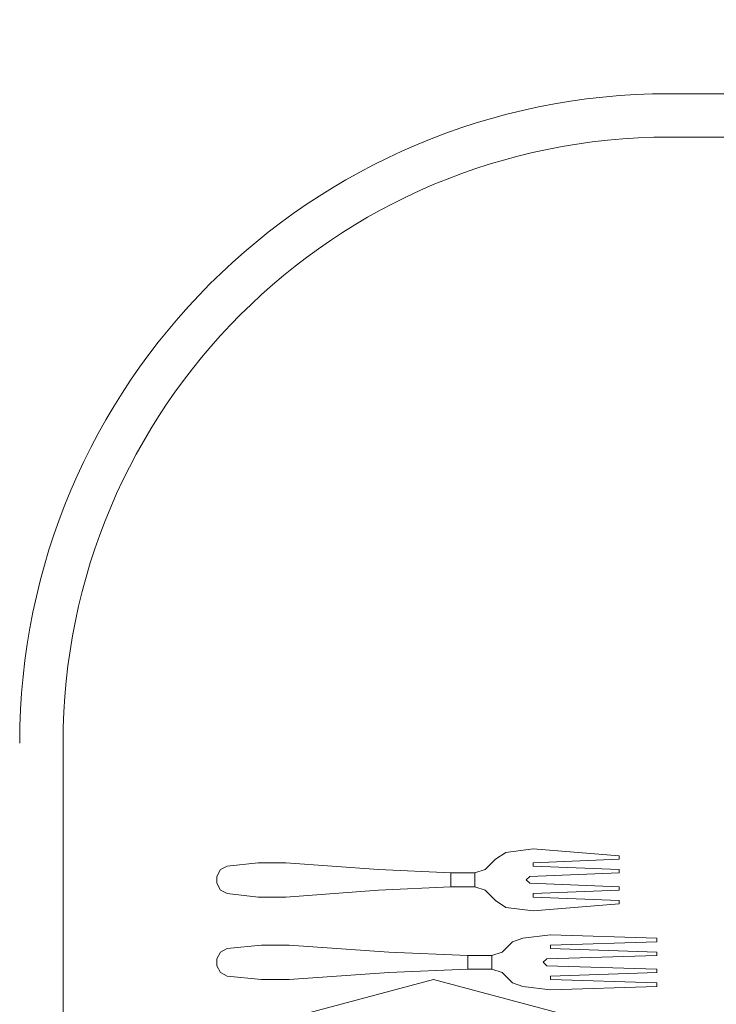
# Model space of a CAD drawing. Units: inches. Extents: x 375 to 1122, y 27 to 1069.
# Tile 46 of 155: x 705.14 to 717.62, y 308.18 to 325.82. Entities that reach past the tile are written whole.
import ezdxf

# ---------------------------------------------------------------- set-up
doc = ezdxf.new("R2010")
doc.units = ezdxf.units.IN
doc.layers.add('A-ANNO-DIMS', color=2, linetype='Continuous', lineweight=18)
doc.layers.add('Furniture', color=30, linetype='Continuous', lineweight=18)
doc.styles.get("Standard").update_dxf_attribs({"font": 'arial.ttf'})
doc.dimstyles.new('ISO-25', dxfattribs={"dimtxt": 12, "dimasz": 2.5, "dimexe": 1.5, "dimexo": 1.5, "dimtad": 1, "dimdec": 1, "dimlunit": 3, "dimtxsty": 'Standard', "dimblk": 'ARCHTICK', "dimcen": 2.5, "dimadec": 0, "dimazin": 0, "dimtfac": 1, "dimtdec": 1, "dimtmove": 0, "dimatfit": 3, "dimfxl": 1.5, "dimfxlon": 1, "dimarcsym": 0})

# ---------------------------------------------------------------- blocks, each defined once
blk = doc.blocks.new('A$C403C54AD')
for p, q in [((0.54488, 0.79569, -0.0006), (0.54488, 1.26108, -0.0006)), ((0.56427, 0.79569, -0.0006), (0.56427, 1.26108, -0.0006)), ((0.92321, 0.73013, -0.02105), (0.92475, 0.72551, -0.02059)), ((0.92321, 0.73013, -0.02413), (0.92475, 0.72551, -0.02367)), ((0.88473, 0.72244, -0.02105), (0.88781, 0.71782, -0.02059)), ((0.88473, 0.72244, -0.02413), (0.88781, 0.71782, -0.02367)), ((0.83575, 0.52421, -0.0006), (1.99923, 0.52421, -0.0006))]:
    blk.add_line(p, q)
for radius in [0.29087, 0.27148]:
    blk.add_arc((0.83575, 0.79569, -0.0006), radius, 180, 270)
for points, invisible_edges in [([(0.92629, 0.74244, -0.02045), (0.92167, 0.74244, -0.02045), (0.92321, 0.79016, -0.01335), (0.92475, 0.79016, -0.01335)], 1), ([(0.92629, 0.74244, -0.02353), (0.92167, 0.74244, -0.02353), (0.92321, 0.79016, -0.01643), (0.92475, 0.79016, -0.01643)], 1), ([(0.93244, 0.74091, -0.0207), (0.92782, 0.74244, -0.02045), (0.92936, 0.79016, -0.01335), (0.9309, 0.79016, -0.01335)], 1), ([(0.93244, 0.74091, -0.02378), (0.92782, 0.74244, -0.02353), (0.92936, 0.79016, -0.01643), (0.9309, 0.79016, -0.01643)], 1), ([(0.94014, 0.74244, -0.02045), (0.93552, 0.74091, -0.0207), (0.93706, 0.79016, -0.01335), (0.9386, 0.79016, -0.01335)], 1), ([(0.94014, 0.74244, -0.02353), (0.93552, 0.74091, -0.02378), (0.93706, 0.79016, -0.01643), (0.9386, 0.79016, -0.01643)], 1), ([(0.94168, 0.74244, -0.02045), (0.9463, 0.74244, -0.02045), (0.94476, 0.79016, -0.01335), (0.94322, 0.79016, -0.01335)], 1), ([(0.94168, 0.74244, -0.02353), (0.9463, 0.74244, -0.02353), (0.94476, 0.79016, -0.01643), (0.94322, 0.79016, -0.01643)], 1), ([(0.88935, 0.73475, -0.02045), (0.88319, 0.73475, -0.02045), (0.88627, 0.77323, -0.01335), (0.88781, 0.77323, -0.01335)], 1), ([(0.88935, 0.73475, -0.02353), (0.88319, 0.73475, -0.02353), (0.88627, 0.77323, -0.01643), (0.88781, 0.77323, -0.01643)], 1), ([(0.8955, 0.73321, -0.0207), (0.89088, 0.73475, -0.02045), (0.89242, 0.77323, -0.01335), (0.89396, 0.77323, -0.01335)], 1), ([(0.8955, 0.73321, -0.02378), (0.89088, 0.73475, -0.02353), (0.89242, 0.77323, -0.01643), (0.89396, 0.77323, -0.01643)], 1), ([(0.9032, 0.73475, -0.02045), (0.89858, 0.73321, -0.0207), (0.90012, 0.77323, -0.01335), (0.90166, 0.77323, -0.01335)], 1), ([(0.9032, 0.73475, -0.02353), (0.89858, 0.73321, -0.02378), (0.90012, 0.77323, -0.01643), (0.90166, 0.77323, -0.01643)], 1), ([(0.90474, 0.73475, -0.02045), (0.91089, 0.73475, -0.02045), (0.90782, 0.77323, -0.01335), (0.90628, 0.77323, -0.01335)], 1), ([(0.90474, 0.73475, -0.02353), (0.91089, 0.73475, -0.02353), (0.90782, 0.77323, -0.01643), (0.90628, 0.77323, -0.01643)], 1), ([(0.92321, 0.73013, -0.02105), (0.92782, 0.74244, -0.02045), (0.92629, 0.74244, -0.02045), (0.92167, 0.74244, -0.02045)], 5), ([(0.92321, 0.73013, -0.02413), (0.92782, 0.74244, -0.02353), (0.92629, 0.74244, -0.02353), (0.92167, 0.74244, -0.02353)], 5), ([(0.92321, 0.73013, -0.02413), (0.92321, 0.73013, -0.02105), (0.92167, 0.74244, -0.02045), (0.92167, 0.74244, -0.02353)], 1), ([(0.92321, 0.73013, -0.02105), (0.93398, 0.73924, -0.02085), (0.93244, 0.74091, -0.0207), (0.92782, 0.74244, -0.02045)], 13), ([(0.92321, 0.73013, -0.02413), (0.93398, 0.73924, -0.02392), (0.93244, 0.74091, -0.02378), (0.92782, 0.74244, -0.02353)], 13), ([(0.94476, 0.73013, -0.02105), (0.93398, 0.73924, -0.02085), (0.93552, 0.74091, -0.0207), (0.94014, 0.74244, -0.02045)], 13), ([(0.94476, 0.73013, -0.02413), (0.93398, 0.73924, -0.02392), (0.93552, 0.74091, -0.02378), (0.94014, 0.74244, -0.02353)], 13), ([(0.94476, 0.73013, -0.02105), (0.94014, 0.74244, -0.02045), (0.94168, 0.74244, -0.02045), (0.9463, 0.74244, -0.02045)], 5), ([(0.94476, 0.73013, -0.02413), (0.94014, 0.74244, -0.02353), (0.94168, 0.74244, -0.02353), (0.9463, 0.74244, -0.02353)], 5), ([(0.94476, 0.73013, -0.02105), (0.94476, 0.73013, -0.02413), (0.9463, 0.74244, -0.02353), (0.9463, 0.74244, -0.02045)], 1), ([(0.94476, 0.73013, -0.02105), (0.93398, 0.73924, -0.02085), (0.92321, 0.73013, -0.02105), (0.94476, 0.73013, -0.02105)], 7), ([(0.94476, 0.73013, -0.02413), (0.93398, 0.73924, -0.02392), (0.92321, 0.73013, -0.02413), (0.94476, 0.73013, -0.02413)], 7), ([(0.88473, 0.72244, -0.02105), (0.89088, 0.73475, -0.02045), (0.88935, 0.73475, -0.02045), (0.88319, 0.73475, -0.02045)], 5), ([(0.88473, 0.72244, -0.02413), (0.89088, 0.73475, -0.02353), (0.88935, 0.73475, -0.02353), (0.88319, 0.73475, -0.02353)], 5), ([(0.88473, 0.72244, -0.02413), (0.88473, 0.72244, -0.02105), (0.88319, 0.73475, -0.02045), (0.88319, 0.73475, -0.02353)], 1), ([(0.88473, 0.72244, -0.02105), (0.89704, 0.73155, -0.02085), (0.8955, 0.73321, -0.0207), (0.89088, 0.73475, -0.02045)], 13), ([(0.88473, 0.72244, -0.02413), (0.89704, 0.73155, -0.02392), (0.8955, 0.73321, -0.02378), (0.89088, 0.73475, -0.02353)], 13), ([(0.90935, 0.72244, -0.02105), (0.89704, 0.73155, -0.02085), (0.89858, 0.73321, -0.0207), (0.9032, 0.73475, -0.02045)], 13), ([(0.90935, 0.72244, -0.02413), (0.89704, 0.73155, -0.02392), (0.89858, 0.73321, -0.02378), (0.9032, 0.73475, -0.02353)], 13), ([(0.90935, 0.72244, -0.02105), (0.9032, 0.73475, -0.02045), (0.90474, 0.73475, -0.02045), (0.91089, 0.73475, -0.02045)], 5), ([(0.90935, 0.72244, -0.02413), (0.9032, 0.73475, -0.02353), (0.90474, 0.73475, -0.02353), (0.91089, 0.73475, -0.02353)], 5), ([(0.90935, 0.72244, -0.02105), (0.90935, 0.72244, -0.02413), (0.91089, 0.73475, -0.02353), (0.91089, 0.73475, -0.02045)], 1), ([(0.90935, 0.72244, -0.02105), (0.89704, 0.73155, -0.02085), (0.88473, 0.72244, -0.02105), (0.90935, 0.72244, -0.02105)], 7), ([(0.90935, 0.72244, -0.02413), (0.89704, 0.73155, -0.02392), (0.88473, 0.72244, -0.02413), (0.90935, 0.72244, -0.02413)], 7), ([(0.94322, 0.72551, -0.02059), (0.92475, 0.72551, -0.02059), (0.92321, 0.73013, -0.02105), (0.94476, 0.73013, -0.02105)], 5), ([(0.94322, 0.72551, -0.02367), (0.92475, 0.72551, -0.02367), (0.92321, 0.73013, -0.02413), (0.94476, 0.73013, -0.02413)], 5), ([(0.92475, 0.72551, -0.02059), (0.92475, 0.72551, -0.02367), (0.92321, 0.73013, -0.02413), (0.92321, 0.73013, -0.02105)], 4), ([(0.94322, 0.72551, -0.02367), (0.94322, 0.72551, -0.02059), (0.94476, 0.73013, -0.02105), (0.94476, 0.73013, -0.02413)], 4), ([(0.92782, 0.72244, -0.02243), (0.94014, 0.72244, -0.02243), (0.94322, 0.72551, -0.02367), (0.92475, 0.72551, -0.02367)], 5), ([(0.92782, 0.72244, -0.01935), (0.94014, 0.72244, -0.01935), (0.94322, 0.72551, -0.02059), (0.92475, 0.72551, -0.02059)], 5), ([(0.90628, 0.71782, -0.02059), (0.88781, 0.71782, -0.02059), (0.88473, 0.72244, -0.02105), (0.90935, 0.72244, -0.02105)], 5), ([(0.90628, 0.71782, -0.02367), (0.88781, 0.71782, -0.02367), (0.88473, 0.72244, -0.02413), (0.90935, 0.72244, -0.02413)], 5), ([(0.88781, 0.71782, -0.02059), (0.88781, 0.71782, -0.02367), (0.88473, 0.72244, -0.02413), (0.88473, 0.72244, -0.02105)], 4), ([(0.90628, 0.71782, -0.02367), (0.90628, 0.71782, -0.02059), (0.90935, 0.72244, -0.02105), (0.90935, 0.72244, -0.02413)], 4), ([(0.92936, 0.7209, -0.0183), (0.9386, 0.7209, -0.0183), (0.94014, 0.72244, -0.01935), (0.92782, 0.72244, -0.01935)], 5), ([(0.92936, 0.7209, -0.02109), (0.9386, 0.7209, -0.02109), (0.94014, 0.72244, -0.02243), (0.92782, 0.72244, -0.02243)], 5), ([(0.92936, 0.7209, -0.0183), (0.92936, 0.7209, -0.02109), (0.92782, 0.72244, -0.02243), (0.92782, 0.72244, -0.01935)], 1), ([(0.93706, 0.71628, -0.01595), (0.9309, 0.71628, -0.01595), (0.92936, 0.7209, -0.0183), (0.9386, 0.7209, -0.0183)], 4), ([(0.9309, 0.71628, -0.01854), (0.9309, 0.71628, -0.01595), (0.92936, 0.7209, -0.0183), (0.92936, 0.7209, -0.02109)], 5), ([(0.93706, 0.71628, -0.01854), (0.9309, 0.71628, -0.01854), (0.92936, 0.7209, -0.02109), (0.9386, 0.7209, -0.02109)], 4), ([(0.93706, 0.71628, -0.01595), (0.93706, 0.71628, -0.01854), (0.9386, 0.7209, -0.02109), (0.9386, 0.7209, -0.0183)], 5), ([(0.9386, 0.7209, -0.02109), (0.9386, 0.7209, -0.0183), (0.94014, 0.72244, -0.01935), (0.94014, 0.72244, -0.02243)], 1), ([(0.89088, 0.71474, -0.02243), (0.9032, 0.71474, -0.02243), (0.90628, 0.71782, -0.02367), (0.88781, 0.71782, -0.02367)], 5), ([(0.89088, 0.71474, -0.01935), (0.9032, 0.71474, -0.01935), (0.90628, 0.71782, -0.02059), (0.88781, 0.71782, -0.02059)], 5), ([(0.89242, 0.7132, -0.0183), (0.90166, 0.7132, -0.0183), (0.9032, 0.71474, -0.01935), (0.89088, 0.71474, -0.01935)], 5), ([(0.89242, 0.7132, -0.02109), (0.90166, 0.7132, -0.02109), (0.9032, 0.71474, -0.02243), (0.89088, 0.71474, -0.02243)], 5), ([(0.89242, 0.7132, -0.0183), (0.89242, 0.7132, -0.02109), (0.89088, 0.71474, -0.02243), (0.89088, 0.71474, -0.01935)], 1), ([(0.90166, 0.7132, -0.02109), (0.90166, 0.7132, -0.0183), (0.9032, 0.71474, -0.01935), (0.9032, 0.71474, -0.02243)], 1), ([(0.9309, 0.71628, -0.01854), (0.9309, 0.71628, -0.01595), (0.9309, 0.7055, -0.01387), (0.9309, 0.7055, -0.01646)], 5), ([(0.93706, 0.7055, -0.01646), (0.93706, 0.7055, -0.01387), (0.93706, 0.71628, -0.01595), (0.93706, 0.71628, -0.01854)], 5), ([(0.90012, 0.70858, -0.01595), (0.89396, 0.70858, -0.01595), (0.89242, 0.7132, -0.0183), (0.90166, 0.7132, -0.0183)], 4), ([(0.90012, 0.70858, -0.01854), (0.89396, 0.70858, -0.01854), (0.89242, 0.7132, -0.02109), (0.90166, 0.7132, -0.02109)], 4), ([(0.89396, 0.70858, -0.01854), (0.89396, 0.70858, -0.01595), (0.89242, 0.7132, -0.0183), (0.89242, 0.7132, -0.02109)], 5), ([(0.90012, 0.70858, -0.01595), (0.90012, 0.70858, -0.01854), (0.90166, 0.7132, -0.02109), (0.90166, 0.7132, -0.0183)], 5), ([(0.89396, 0.70858, -0.01854), (0.89396, 0.70858, -0.01595), (0.89396, 0.69781, -0.01387), (0.89396, 0.69781, -0.01646)], 5), ([(0.90012, 0.69781, -0.01646), (0.90012, 0.69781, -0.01387), (0.90012, 0.70858, -0.01595), (0.90012, 0.70858, -0.01854)], 5), ([(0.9386, 0.6701, -0.01678), (0.92936, 0.6701, -0.01678), (0.9309, 0.7055, -0.01387), (0.93706, 0.7055, -0.01387)], 1), ([(0.9309, 0.7055, -0.01387), (0.9309, 0.7055, -0.01646), (0.92936, 0.6701, -0.01986), (0.92936, 0.6701, -0.01678)], 5), ([(0.9386, 0.6701, -0.01986), (0.92936, 0.6701, -0.01986), (0.9309, 0.7055, -0.01646), (0.93706, 0.7055, -0.01646)], 1), ([(0.9386, 0.6701, -0.01678), (0.9386, 0.6701, -0.01986), (0.93706, 0.7055, -0.01646), (0.93706, 0.7055, -0.01387)], 5), ([(0.90166, 0.66549, -0.01678), (0.89242, 0.66549, -0.01678), (0.89396, 0.69781, -0.01387), (0.90012, 0.69781, -0.01387)], 1), ([(0.89396, 0.69781, -0.01387), (0.89396, 0.69781, -0.01646), (0.89242, 0.66549, -0.01986), (0.89242, 0.66549, -0.01678)], 5), ([(0.90166, 0.66549, -0.01986), (0.89242, 0.66549, -0.01986), (0.89396, 0.69781, -0.01646), (0.90012, 0.69781, -0.01646)], 1), ([(0.90166, 0.66549, -0.01678), (0.90166, 0.66549, -0.01986), (0.90012, 0.69781, -0.01646), (0.90012, 0.69781, -0.01387)], 5), ([(0.92629, 0.62547, -0.01916), (0.94168, 0.62547, -0.01916), (0.9386, 0.6701, -0.01678), (0.92936, 0.6701, -0.01678)], 5), ([(0.92629, 0.62547, -0.0238), (0.94168, 0.62547, -0.0238), (0.9386, 0.6701, -0.01986), (0.92936, 0.6701, -0.01986)], 5), ([(0.92936, 0.6701, -0.01986), (0.92936, 0.6701, -0.01678), (0.92629, 0.62547, -0.01916), (0.92629, 0.62547, -0.0238)], 1), ([(0.94168, 0.62547, -0.0238), (0.94168, 0.62547, -0.01916), (0.9386, 0.6701, -0.01678), (0.9386, 0.6701, -0.01986)], 4), ([(0.88935, 0.62393, -0.01916), (0.90474, 0.62393, -0.01916), (0.90166, 0.66549, -0.01678), (0.89242, 0.66549, -0.01678)], 5), ([(0.88935, 0.62393, -0.0238), (0.90474, 0.62393, -0.0238), (0.90166, 0.66549, -0.01986), (0.89242, 0.66549, -0.01986)], 5), ([(0.89242, 0.66549, -0.01986), (0.89242, 0.66549, -0.01678), (0.88935, 0.62393, -0.01916), (0.88935, 0.62393, -0.0238)], 1), ([(0.90474, 0.62393, -0.0238), (0.90474, 0.62393, -0.01916), (0.90166, 0.66549, -0.01678), (0.90166, 0.66549, -0.01986)], 4), ([(0.90474, 0.61161, -0.01949), (0.88935, 0.61161, -0.01949), (0.88935, 0.62393, -0.01916), (0.90474, 0.62393, -0.01916)], 5), ([(0.90474, 0.61161, -0.02413), (0.88935, 0.61161, -0.02413), (0.88935, 0.62393, -0.0238), (0.90474, 0.62393, -0.0238)], 5), ([(0.94168, 0.61315, -0.01949), (0.92629, 0.61315, -0.01949), (0.92629, 0.62547, -0.01916), (0.94168, 0.62547, -0.01916)], 5), ([(0.94168, 0.61315, -0.02413), (0.92629, 0.61315, -0.02413), (0.92629, 0.62547, -0.0238), (0.94168, 0.62547, -0.0238)], 5), ([(0.92782, 0.59776, -0.01946), (0.94014, 0.59776, -0.01946), (0.94168, 0.61315, -0.01949), (0.92629, 0.61315, -0.01949)], 5), ([(0.92782, 0.59776, -0.02409), (0.94014, 0.59776, -0.02409), (0.94168, 0.61315, -0.02413), (0.92629, 0.61315, -0.02413)], 5), ([(0.89088, 0.59776, -0.01946), (0.9032, 0.59776, -0.01946), (0.90474, 0.61161, -0.01949), (0.88935, 0.61161, -0.01949)], 5), ([(0.89088, 0.59776, -0.02409), (0.9032, 0.59776, -0.02409), (0.90474, 0.61161, -0.02413), (0.88935, 0.61161, -0.02413)], 5), ([(0.90166, 0.59468, -0.01921), (0.89242, 0.59468, -0.01921), (0.89088, 0.59776, -0.01946), (0.9032, 0.59776, -0.01946)], 5), ([(0.90166, 0.59468, -0.02385), (0.89242, 0.59468, -0.02385), (0.89088, 0.59776, -0.02409), (0.9032, 0.59776, -0.02409)], 5), ([(0.9386, 0.59468, -0.01921), (0.92936, 0.59468, -0.01921), (0.92782, 0.59776, -0.01946), (0.94014, 0.59776, -0.01946)], 5), ([(0.9386, 0.59468, -0.02385), (0.92936, 0.59468, -0.02385), (0.92782, 0.59776, -0.02409), (0.94014, 0.59776, -0.02409)], 5), ([(0.8955, 0.59314, -0.01938), (0.89858, 0.59314, -0.01938), (0.90166, 0.59468, -0.01921), (0.89242, 0.59468, -0.01921)], 4), ([(0.8955, 0.59314, -0.02351), (0.89858, 0.59314, -0.02351), (0.90166, 0.59468, -0.02385), (0.89242, 0.59468, -0.02385)], 4), ([(0.93244, 0.59314, -0.01938), (0.93552, 0.59314, -0.01938), (0.9386, 0.59468, -0.01921), (0.92936, 0.59468, -0.01921)], 4), ([(0.93244, 0.59314, -0.02351), (0.93552, 0.59314, -0.02351), (0.9386, 0.59468, -0.02385), (0.92936, 0.59468, -0.02385)], 4)]:
    blk.add_3dface(points, dxfattribs=dict(invisible_edges=invisible_edges))
for points in [[(0.92321, 0.79016, -0.01335), (0.92321, 0.79016, -0.01643), (0.92167, 0.74244, -0.02353), (0.92167, 0.74244, -0.02045)], [(0.92475, 0.79016, -0.01643), (0.92475, 0.79016, -0.01335), (0.92321, 0.79016, -0.01335), (0.92321, 0.79016, -0.01643)], [(0.92629, 0.74244, -0.02045), (0.92629, 0.74244, -0.02353), (0.92475, 0.79016, -0.01643), (0.92475, 0.79016, -0.01335)], [(0.92936, 0.79016, -0.01335), (0.92936, 0.79016, -0.01643), (0.92782, 0.74244, -0.02353), (0.92782, 0.74244, -0.02045)], [(0.9309, 0.79016, -0.01643), (0.9309, 0.79016, -0.01335), (0.92936, 0.79016, -0.01335), (0.92936, 0.79016, -0.01643)], [(0.93244, 0.74091, -0.02378), (0.93244, 0.74091, -0.0207), (0.9309, 0.79016, -0.01335), (0.9309, 0.79016, -0.01643)], [(0.93706, 0.79016, -0.01643), (0.93706, 0.79016, -0.01335), (0.93552, 0.74091, -0.0207), (0.93552, 0.74091, -0.02378)], [(0.9386, 0.79016, -0.01643), (0.9386, 0.79016, -0.01335), (0.93706, 0.79016, -0.01335), (0.93706, 0.79016, -0.01643)], [(0.94014, 0.74244, -0.02353), (0.94014, 0.74244, -0.02045), (0.9386, 0.79016, -0.01335), (0.9386, 0.79016, -0.01643)], [(0.94322, 0.79016, -0.01335), (0.94322, 0.79016, -0.01643), (0.94168, 0.74244, -0.02353), (0.94168, 0.74244, -0.02045)], [(0.94476, 0.79016, -0.01643), (0.94476, 0.79016, -0.01335), (0.94322, 0.79016, -0.01335), (0.94322, 0.79016, -0.01643)], [(0.9463, 0.74244, -0.02353), (0.9463, 0.74244, -0.02045), (0.94476, 0.79016, -0.01335), (0.94476, 0.79016, -0.01643)], [(0.88627, 0.77323, -0.01335), (0.88627, 0.77323, -0.01643), (0.88319, 0.73475, -0.02353), (0.88319, 0.73475, -0.02045)], [(0.88781, 0.77323, -0.01643), (0.88781, 0.77323, -0.01335), (0.88627, 0.77323, -0.01335), (0.88627, 0.77323, -0.01643)], [(0.88935, 0.73475, -0.02045), (0.88935, 0.73475, -0.02353), (0.88781, 0.77323, -0.01643), (0.88781, 0.77323, -0.01335)], [(0.89242, 0.77323, -0.01335), (0.89242, 0.77323, -0.01643), (0.89088, 0.73475, -0.02353), (0.89088, 0.73475, -0.02045)], [(0.89396, 0.77323, -0.01643), (0.89396, 0.77323, -0.01335), (0.89242, 0.77323, -0.01335), (0.89242, 0.77323, -0.01643)], [(0.8955, 0.73321, -0.02378), (0.8955, 0.73321, -0.0207), (0.89396, 0.77323, -0.01335), (0.89396, 0.77323, -0.01643)], [(0.90012, 0.77323, -0.01643), (0.90012, 0.77323, -0.01335), (0.89858, 0.73321, -0.0207), (0.89858, 0.73321, -0.02378)], [(0.90166, 0.77323, -0.01643), (0.90166, 0.77323, -0.01335), (0.90012, 0.77323, -0.01335), (0.90012, 0.77323, -0.01643)], [(0.9032, 0.73475, -0.02353), (0.9032, 0.73475, -0.02045), (0.90166, 0.77323, -0.01335), (0.90166, 0.77323, -0.01643)], [(0.90628, 0.77323, -0.01335), (0.90628, 0.77323, -0.01643), (0.90474, 0.73475, -0.02353), (0.90474, 0.73475, -0.02045)], [(0.90782, 0.77323, -0.01643), (0.90782, 0.77323, -0.01335), (0.90628, 0.77323, -0.01335), (0.90628, 0.77323, -0.01643)], [(0.91089, 0.73475, -0.02353), (0.91089, 0.73475, -0.02045), (0.90782, 0.77323, -0.01335), (0.90782, 0.77323, -0.01643)], [(0.92629, 0.74244, -0.02045), (0.92629, 0.74244, -0.02353), (0.92782, 0.74244, -0.02353), (0.92782, 0.74244, -0.02045)], [(0.94014, 0.74244, -0.02353), (0.94014, 0.74244, -0.02045), (0.94168, 0.74244, -0.02045), (0.94168, 0.74244, -0.02353)], [(0.93244, 0.74091, -0.0207), (0.93244, 0.74091, -0.02378), (0.93398, 0.73924, -0.02392), (0.93398, 0.73924, -0.02085)], [(0.93398, 0.73924, -0.02392), (0.93398, 0.73924, -0.02085), (0.93552, 0.74091, -0.0207), (0.93552, 0.74091, -0.02378)], [(0.88935, 0.73475, -0.02045), (0.88935, 0.73475, -0.02353), (0.89088, 0.73475, -0.02353), (0.89088, 0.73475, -0.02045)], [(0.8955, 0.73321, -0.0207), (0.8955, 0.73321, -0.02378), (0.89704, 0.73155, -0.02392), (0.89704, 0.73155, -0.02085)], [(0.89704, 0.73155, -0.02392), (0.89704, 0.73155, -0.02085), (0.89858, 0.73321, -0.0207), (0.89858, 0.73321, -0.02378)], [(0.9032, 0.73475, -0.02353), (0.9032, 0.73475, -0.02045), (0.90474, 0.73475, -0.02045), (0.90474, 0.73475, -0.02353)], [(0.92782, 0.72244, -0.02243), (0.92782, 0.72244, -0.01935), (0.92475, 0.72551, -0.02059), (0.92475, 0.72551, -0.02367)], [(0.94014, 0.72244, -0.01935), (0.94014, 0.72244, -0.02243), (0.94322, 0.72551, -0.02367), (0.94322, 0.72551, -0.02059)], [(0.89088, 0.71474, -0.02243), (0.89088, 0.71474, -0.01935), (0.88781, 0.71782, -0.02059), (0.88781, 0.71782, -0.02367)], [(0.9032, 0.71474, -0.01935), (0.9032, 0.71474, -0.02243), (0.90628, 0.71782, -0.02367), (0.90628, 0.71782, -0.02059)], [(0.9309, 0.7055, -0.01387), (0.93706, 0.7055, -0.01387), (0.93706, 0.71628, -0.01595), (0.9309, 0.71628, -0.01595)], [(0.9309, 0.7055, -0.01646), (0.93706, 0.7055, -0.01646), (0.93706, 0.71628, -0.01854), (0.9309, 0.71628, -0.01854)], [(0.89396, 0.69781, -0.01387), (0.90012, 0.69781, -0.01387), (0.90012, 0.70858, -0.01595), (0.89396, 0.70858, -0.01595)], [(0.89396, 0.69781, -0.01646), (0.90012, 0.69781, -0.01646), (0.90012, 0.70858, -0.01854), (0.89396, 0.70858, -0.01854)], [(0.88935, 0.62393, -0.01916), (0.88935, 0.62393, -0.0238), (0.88935, 0.61161, -0.02413), (0.88935, 0.61161, -0.01949)], [(0.90474, 0.61161, -0.01949), (0.90474, 0.61161, -0.02413), (0.90474, 0.62393, -0.0238), (0.90474, 0.62393, -0.01916)], [(0.92629, 0.62547, -0.01916), (0.92629, 0.62547, -0.0238), (0.92629, 0.61315, -0.02413), (0.92629, 0.61315, -0.01949)], [(0.94168, 0.61315, -0.01949), (0.94168, 0.61315, -0.02413), (0.94168, 0.62547, -0.0238), (0.94168, 0.62547, -0.01916)], [(0.92629, 0.61315, -0.02413), (0.92629, 0.61315, -0.01949), (0.92782, 0.59776, -0.01946), (0.92782, 0.59776, -0.02409)], [(0.94014, 0.59776, -0.02409), (0.94014, 0.59776, -0.01946), (0.94168, 0.61315, -0.01949), (0.94168, 0.61315, -0.02413)], [(0.88935, 0.61161, -0.02413), (0.88935, 0.61161, -0.01949), (0.89088, 0.59776, -0.01946), (0.89088, 0.59776, -0.02409)], [(0.9032, 0.59776, -0.02409), (0.9032, 0.59776, -0.01946), (0.90474, 0.61161, -0.01949), (0.90474, 0.61161, -0.02413)], [(0.89088, 0.59776, -0.01946), (0.89088, 0.59776, -0.02409), (0.89242, 0.59468, -0.02385), (0.89242, 0.59468, -0.01921)], [(0.90166, 0.59468, -0.01921), (0.90166, 0.59468, -0.02385), (0.9032, 0.59776, -0.02409), (0.9032, 0.59776, -0.01946)], [(0.92782, 0.59776, -0.01946), (0.92782, 0.59776, -0.02409), (0.92936, 0.59468, -0.02385), (0.92936, 0.59468, -0.01921)], [(0.9386, 0.59468, -0.01921), (0.9386, 0.59468, -0.02385), (0.94014, 0.59776, -0.02409), (0.94014, 0.59776, -0.01946)], [(0.89242, 0.59468, -0.02385), (0.89242, 0.59468, -0.01921), (0.8955, 0.59314, -0.01938), (0.8955, 0.59314, -0.02351)], [(0.8955, 0.59314, -0.01938), (0.8955, 0.59314, -0.02351), (0.89858, 0.59314, -0.02351), (0.89858, 0.59314, -0.01938)], [(0.89858, 0.59314, -0.02351), (0.89858, 0.59314, -0.01938), (0.90166, 0.59468, -0.01921), (0.90166, 0.59468, -0.02385)], [(0.92936, 0.59468, -0.02385), (0.92936, 0.59468, -0.01921), (0.93244, 0.59314, -0.01938), (0.93244, 0.59314, -0.02351)], [(0.93244, 0.59314, -0.01938), (0.93244, 0.59314, -0.02351), (0.93552, 0.59314, -0.02351), (0.93552, 0.59314, -0.01938)], [(0.93552, 0.59314, -0.02351), (0.93552, 0.59314, -0.01938), (0.9386, 0.59468, -0.01921), (0.9386, 0.59468, -0.02385)]]:
    blk.add_3dface(points)
at = {"linetype": 'ByBlock', "invisible_edges": 5}
for points in [[(0.96024, 0.75938, -0.00874), (0.97623, 0.75014, -0.00874), (0.96015, 0.69011, -0.00874), (0.94168, 0.69011, -0.00874)], [(0.98956, 0.74244, -0.02259), (0.96024, 0.75938, -0.01335), (0.94168, 0.69011, -0.01335), (0.97554, 0.69011, -0.02259)], [(0.94168, 0.69011, -0.00874), (0.96015, 0.69011, -0.00874), (0.97623, 0.63008, -0.00874), (0.96024, 0.62085, -0.00874)], [(0.97554, 0.69011, -0.02259), (0.94168, 0.69011, -0.01335), (0.96024, 0.62085, -0.01335), (0.98956, 0.63778, -0.02259)]]:
    blk.add_3dface(points, dxfattribs=at)
at = {"linetype": 'ByBlock'}
for points in [[(0.96024, 0.75938, -0.01335), (0.96024, 0.75938, -0.00874), (0.94168, 0.69011, -0.00874), (0.94168, 0.69011, -0.01335)], [(0.94168, 0.69011, -0.01335), (0.94168, 0.69011, -0.00874), (0.96024, 0.62085, -0.00874), (0.96024, 0.62085, -0.01335)]]:
    blk.add_3dface(points, dxfattribs=at)
blk = doc.blocks.new('_ArchTick')
at = {"color": 0, "linetype": 'ByBlock', "const_width": 0.15}
blk.add_lwpolyline([(-0.5, -0.5), (0.5, 0.5)], dxfattribs=at)
blk = doc.blocks.new('*D59')
at = {"layer": 'A-ANNO-DIMS', "color": 0, "lineweight": -2, "transparency": 16777216}
for p, q in [((668.717, 346.851), (665.717, 346.851)), ((667.217, 346.851), (667.217, 232.348)), ((668.717, 232.348), (665.717, 232.348)), ((667.217, 232.348), (667.217, 27.496))]:
    blk.add_line(p, q, dxfattribs=at)
at = {"layer": 'Defpoints', "color": 0, "transparency": 16777216}
for p in [(684.392, 346.851), (667.217, 232.348), (684.392, 232.348)]:
    blk.add_point(p, dxfattribs=at)
at = {"layer": 'A-ANNO-DIMS', "color": 0, "lineweight": -2, "transparency": 16777216, "xscale": 2.5, "yscale": 2.5, "zscale": 2.5}
for p, rotation in [((667.217, 346.851), 90), ((667.217, 232.348), 270)]:
    blk.add_blockref('_ArchTick', p, dxfattribs=dict(at, rotation=rotation))
at = {"layer": 'A-ANNO-DIMS', "color": 0, "transparency": 16777216, "insert": (660.387, 128.672), "char_height": 12, "attachment_point": 5, "rotation": 90}
blk.add_mtext('DINING SET 9\'-6 1/2" TYP.', dxfattribs=at)

msp = doc.modelspace()

# ---------------------------------------------------------------- block references
at = {"layer": 'Furniture', "xscale": 39.9918517141215, "yscale": 39.9918517141215, "zscale": 39.9918517141215, "rotation": 270}
msp.add_blockref('A$C403C54AD', (684.955, 346.287, 0.024), dxfattribs=at)

# ---------------------------------------------------------------- dimensions: what is measured, and where the dimension line sits
at = {"layer": 'A-ANNO-DIMS'}
dim = msp.add_linear_dim(base=(667.217, 232.348), p1=(684.392, 346.851), p2=(684.392, 232.348), angle=270, text='DINING SET <> TYP.', dimstyle='ISO-25', override={"dimdec": 1, "dimlfac": 1, "dimrnd": 0, "dimzin": 1, "dimdsep": 46, "dimlunit": 4, "dimfrac": 2}, dxfattribs=at)
dim.commit()
dim.dimension.update_dxf_attribs({"geometry": '*D59', "text_midpoint": (660.387, 128.672)})

doc.saveas('drawing.dxf')
